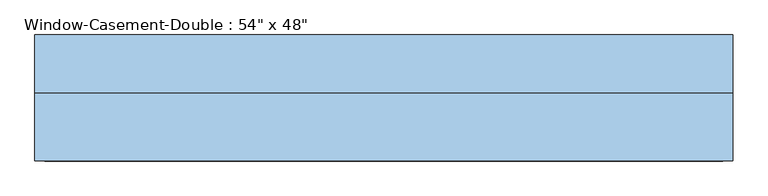
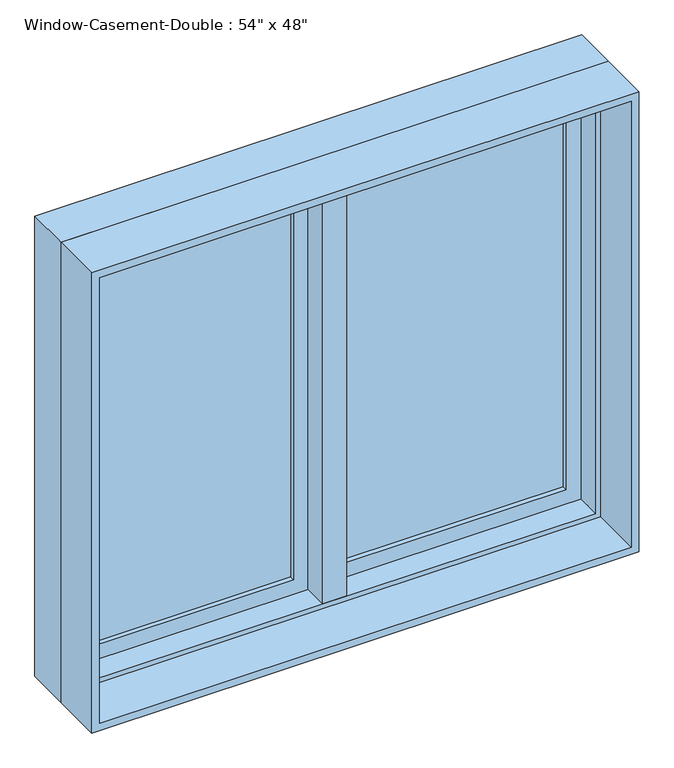
"""IFC4 building model written with IfcOpenShell, lengths in millimetres: window geometry."""

from ifc_helpers import new_model, si_unit, frame, origin, place, context, project, spatial, polyline, outline, extrude, faceted_brep, source, transform, mapped, element, save


def window_ecc443c5(model_context):
    return source(origin(), model_context, "Body", "SolidModel", [
        faceted_brep([(9.525, 133.35, 2120.9), (-9.525, 133.35, 2120.9), (-9.525, 82.55, 2120.9), (9.525, 82.55, 2120.9), (9.525, 133.35, 927.1), (9.525, 82.55, 927.1), (-9.525, 82.55, 927.1), (-9.525, 133.35, 927.1), (-9.525, 82.55, 946.15), (-9.525, 82.55, 2101.85), (-30.1625, 82.55, 946.15), (-30.1625, 82.55, 2101.85), (-30.1625, 19.05, 946.15), (-30.1625, 19.05, 2101.85), (30.1625, 19.05, 946.15), (30.1625, 19.05, 2101.85), (30.1625, 82.55, 946.15), (30.1625, 82.55, 2101.85), (9.525, 82.55, 946.15), (9.525, 82.55, 2101.85)], [[[0, 1, 2, 3]], [[4, 5, 6, 7]], [[1, 0, 4, 7]], [[2, 1, 7, 6, 8, 9]], [[9, 8, 10, 11]], [[11, 10, 12, 13]], [[13, 12, 14, 15]], [[15, 14, 16, 17]], [[17, 16, 18, 19]], [[0, 3, 19, 18, 5, 4]], [[18, 8, 6, 5]], [[9, 19, 3, 2]], [[8, 18, 16, 14, 12, 10]], [[19, 9, 11, 13, 15, 17]]]),
        extrude(outline(polyline([(-66.675, 114.3), (-66.675, 107.95), (-615.95, 107.95), (-615.95, 114.3), (-66.675, 114.3)])), frame((0.0, 0.0, 984.25), z_axis=(0.0, 0.0, 1.0), x_axis=(1.0, 0.0, 0.0)), (0.0, 0.0, 1.0), 1079.5),
        extrude(outline(polyline([(-615.95, 95.25), (-615.95, 101.6), (-66.675, 101.6), (-66.675, 95.25), (-615.95, 95.25)])), frame((0.0, 0.0, 984.25), z_axis=(0.0, 0.0, 1.0), x_axis=(1.0, 0.0, 0.0)), (0.0, 0.0, 1.0), 1079.5),
        extrude(outline(polyline([(615.95, 114.3), (615.95, 107.95), (66.675, 107.95), (66.675, 114.3), (615.95, 114.3)])), frame((0.0, 0.0, 984.25), z_axis=(0.0, 0.0, 1.0), x_axis=(1.0, 0.0, 0.0)), (0.0, 0.0, 1.0), 1079.5),
        extrude(outline(polyline([(66.675, 95.25), (66.675, 101.6), (615.95, 101.6), (615.95, 95.25), (66.675, 95.25)])), frame((0.0, 0.0, 984.25), z_axis=(0.0, 0.0, 1.0), x_axis=(1.0, 0.0, 0.0)), (0.0, 0.0, 1.0), 1079.5),
        extrude(outline(polyline([(2120.9, -673.1), (927.1, -673.1), (927.1, -9.525), (2120.9, -9.525), (2120.9, -673.1)]), holes=[polyline([(2063.75, -66.675), (984.25, -66.675), (984.25, -615.95), (2063.75, -615.95), (2063.75, -66.675)])]), frame((0.0, 82.55, 0.0), z_axis=(0.0, 1.0, 0.0), x_axis=(0.0, 0.0, 1.0)), (0.0, 0.0, 1.0), 44.45),
        extrude(outline(polyline([(927.1, 673.1), (2120.9, 673.1), (2120.9, 9.525), (927.1, 9.525), (927.1, 673.1)]), holes=[polyline([(984.25, 66.675), (2063.75, 66.675), (2063.75, 615.95), (984.25, 615.95), (984.25, 66.675)])]), frame((0.0, 82.55, 0.0), z_axis=(0.0, 1.0, 0.0), x_axis=(0.0, 0.0, 1.0)), (0.0, 0.0, 1.0), 44.45),
        extrude(outline(polyline([(2133.6, -685.8), (914.4, -685.8), (914.4, 685.8), (2133.6, 685.8), (2133.6, -685.8)]), holes=[polyline([(2114.55, 666.75), (933.45, 666.75), (933.45, -666.75), (2114.55, -666.75), (2114.55, 666.75)])]), frame((0.0, -114.3, 0.0), z_axis=(0.0, 1.0, 0.0), x_axis=(0.0, 0.0, 1.0)), (0.0, 0.0, 1.0), 133.35),
        faceted_brep([(654.05, 82.55, 2101.85), (654.05, 19.05, 2101.85), (-654.05, 19.05, 2101.85), (-654.05, 82.55, 2101.85), (673.1, 133.35, 2120.9), (673.1, 82.55, 2120.9), (-673.1, 82.55, 2120.9), (-673.1, 133.35, 2120.9), (685.8, 19.05, 2133.6), (685.8, 133.35, 2133.6), (-685.8, 133.35, 2133.6), (-685.8, 19.05, 2133.6), (-654.05, 19.05, 946.15), (-654.05, 82.55, 946.15), (-673.1, 82.55, 927.1), (-673.1, 133.35, 927.1), (-685.8, 133.35, 914.4), (-685.8, 19.05, 914.4), (654.05, 19.05, 946.15), (654.05, 82.55, 946.15), (673.1, 82.55, 927.1), (673.1, 133.35, 927.1), (685.8, 133.35, 914.4), (685.8, 19.05, 914.4)], [[[0, 1, 2, 3]], [[4, 5, 6, 7]], [[8, 9, 10, 11]], [[3, 2, 12, 13]], [[7, 6, 14, 15]], [[11, 10, 16, 17]], [[13, 12, 18, 19]], [[15, 14, 20, 21]], [[17, 16, 22, 23]], [[11, 17, 23, 8], [1, 18, 12, 2]], [[19, 18, 1, 0]], [[5, 20, 14, 6], [3, 13, 19, 0]], [[21, 20, 5, 4]], [[23, 22, 9, 8]], [[9, 22, 16, 10], [7, 15, 21, 4]]]),
    ])


if __name__ == "__main__":
    model = new_model("IFC4")
    model_context = context("Model", 3, world=origin())
    ifc_project = project(units=[si_unit("LENGTHUNIT", "METRE", prefix="MILLI")], contexts=[model_context])
    site = spatial("IfcSite", under=ifc_project)
    building = spatial("IfcBuilding", under=site)
    placement = place(None, origin())
    window_shape = window_ecc443c5(model_context)
    element("IfcWindow", 1, ObjectType="Window-Casement-Double : 54\" x 48\"", at=placement, inside=building, context=model_context, shape_type="MappedRepresentation", body=[
        mapped(window_shape, transform((0.0, 0.0, 0.0), x_axis=(1.0, 0.0, 0.0), y_axis=(0.0, 1.0, 0.0), z_axis=(0.0, 0.0, 1.0))),
    ])
    save(model, "model.ifc")

# Revit data of these elements
# Type "Window-Casement-Double : 54\" x 48\""
#   Type Mark = "19"
#   Fire Rating = "0.5h"
#   Assembly Code = "B2020100"
#   Analytic Construction = "Double glazing - domestic"
#   Frame Extension [instance default] = 0' - 0 1/4"
#   Window Inset [instance default] = 0' - 0"
#   Wall Thickness [instance default] = 0' - 6"
#   Interior Wall Closure [instance default] = 0' - 2 1/4"
#   Half Width = 2' - 3"
#   Visual Light Transmittance = 0.81
#   Thermal Resistance (R) = 1.8146 (h·ft²·°F)/BTU
#   Solar Heat Gain Coefficient = 0.76
#   Rough Width = 4' - 6 1/2"
#   Rough Height = 4' - 0 1/2"
#   Height = 4' - 0"
#   Heat Transfer Coefficient (U) = 0.5511 BTU/(h·ft²·°F)
#   Exterior Wall Closure [instance default] = 0' - 1 1/4"
#   Extension Jamb [instance default] = 0' - 2 1/4"
#   Default Sill Height = 3' - 0"
#   Width = 4' - 6"
#   Muntin Visibility = yes
#   Interior Trim Visibility [instance default] = yes
#   Exterior Trim Visibility [instance default] = yes
#   Extension Jamb Visibility [instance default] = yes
#   Interior Trim Material = Wood - Stained
#   Muntin Pattern = Muntin Pattern_2x2 : Muntin Pattern_2x2
#   Interior Trim = Trim-Window-Interior-Flat : Picture Frame
#   Interior Frame Material = Wood - Stained
#   Glass Panel Material = Glass
#   Exterior Trim Material = Clad - White
#   Exterior Trim = Trim-Window-Exterior-Flat : with Sill
#   Exterior Frame Material = Clad - White
#   Wall Closure = (empty or 0)
# Element 1 (IfcWindow, "Window-Casement-Double : 54\" x 48\"")
#   Wall Thickness = 0' - 9"
#   Extension Jamb = 0' - 5 1/4"
#   Materials on its faces: "Wood - Stained", "Glass", "Clad - White"
# Materials
#   "Wood - Stained": class "Wood", colour RGB 224 178 126, transparency 0, Cost = 0
#   "Glass": class "Glass", colour RGB 0 128 192, transparency 0.75, Description = "Soda Lime Glass", Cost = 0
#   "Clad - White": class "Wood", colour RGB 242 242 238, transparency 0, Cost = 0
